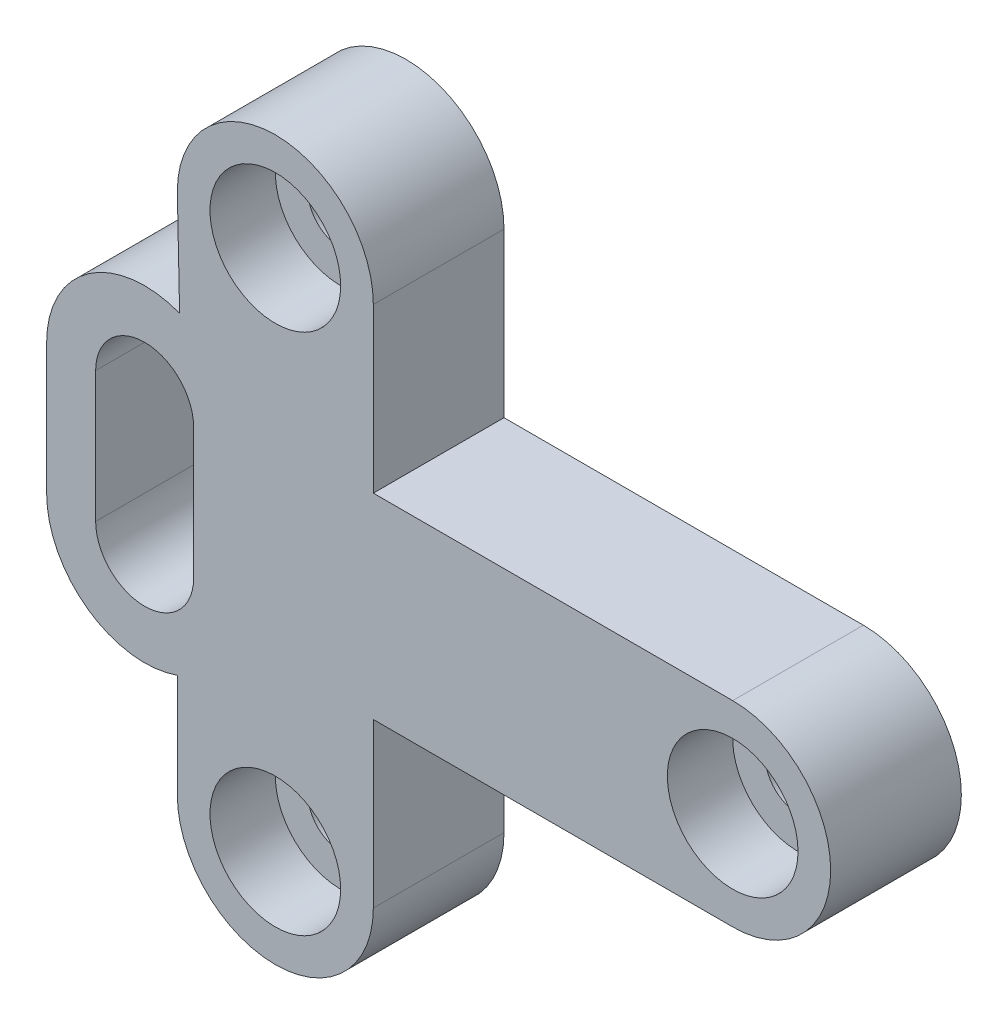
ISO-10303-21;
HEADER;
FILE_DESCRIPTION(('STEP AP214'),'2;1');
FILE_NAME('part.step','',(''),(''),'','','');
FILE_SCHEMA(('AUTOMOTIVE_DESIGN { 1 0 10303 214 1 1 1 1 }'));
ENDSEC;
DATA;
#1=APPLICATION_CONTEXT('core data for automotive mechanical design processes');
#2=APPLICATION_PROTOCOL_DEFINITION('international standard','automotive_design',2000,#1);
#3=PRODUCT_CONTEXT('',#1,'mechanical');
#4=PRODUCT('Part','Part','',(#3));
#5=PRODUCT_RELATED_PRODUCT_CATEGORY('part','',(#4));
#6=PRODUCT_DEFINITION_FORMATION('','',#4);
#7=PRODUCT_DEFINITION_CONTEXT('part definition',#1,'design');
#8=PRODUCT_DEFINITION('design','',#6,#7);
#9=PRODUCT_DEFINITION_SHAPE('','',#8);
#10=(LENGTH_UNIT() NAMED_UNIT(*) SI_UNIT(.MILLI.,.METRE.));
#11=(NAMED_UNIT(*) PLANE_ANGLE_UNIT() SI_UNIT($,.RADIAN.));
#12=(NAMED_UNIT(*) SI_UNIT($,.STERADIAN.) SOLID_ANGLE_UNIT());
#13=UNCERTAINTY_MEASURE_WITH_UNIT(LENGTH_MEASURE(1.E-05),#10,'distance_accuracy_value','');
#14=(GEOMETRIC_REPRESENTATION_CONTEXT(3) GLOBAL_UNCERTAINTY_ASSIGNED_CONTEXT((#13)) GLOBAL_UNIT_ASSIGNED_CONTEXT((#10,
#11,#12)) REPRESENTATION_CONTEXT('',''));
#15=CARTESIAN_POINT('',(0.,0.,0.));
#16=DIRECTION('',(0.,0.,1.));
#17=DIRECTION('',(1.,0.,0.));
#18=AXIS2_PLACEMENT_3D('',#15,#16,#17);
#19=CARTESIAN_POINT('',(-35.0000000000002,-5.34294830600858E-13,20.));
#20=DIRECTION('',(1.,0.,0.));
#21=DIRECTION('',(0.,1.,0.));
#22=AXIS2_PLACEMENT_3D('',#19,#20,#21);
#23=PLANE('',#22);
#24=DIRECTION('',(0.,-1.,0.));
#25=VECTOR('',#24,1.);
#26=CARTESIAN_POINT('',(-35.0000000000002,-5.34294830600858E-13,0.));
#27=LINE('',#26,#25);
#28=CARTESIAN_POINT('',(-35.0000000000003,10.,0.));
#29=VERTEX_POINT('',#28);
#30=CARTESIAN_POINT('',(-35.,-10.,0.));
#31=VERTEX_POINT('',#30);
#32=EDGE_CURVE('E208',#29,#31,#27,.T.);
#33=ORIENTED_EDGE('',*,*,#32,.T.);
#34=DIRECTION('',(0.,0.,-1.));
#35=VECTOR('',#34,1.);
#36=CARTESIAN_POINT('',(-35.,-10.,20.));
#37=LINE('',#36,#35);
#38=CARTESIAN_POINT('',(-35.,-10.,20.));
#39=VERTEX_POINT('',#38);
#40=EDGE_CURVE('E11',#39,#31,#37,.T.);
#41=ORIENTED_EDGE('',*,*,#40,.F.);
#42=DIRECTION('',(0.,-1.,0.));
#43=VECTOR('',#42,1.);
#44=CARTESIAN_POINT('',(-35.0000000000002,-5.34294830600858E-13,20.));
#45=LINE('',#44,#43);
#46=CARTESIAN_POINT('',(-35.0000000000003,10.,20.));
#47=VERTEX_POINT('',#46);
#48=EDGE_CURVE('E278',#47,#39,#45,.T.);
#49=ORIENTED_EDGE('',*,*,#48,.F.);
#50=DIRECTION('',(0.,0.,-1.));
#51=VECTOR('',#50,1.);
#52=CARTESIAN_POINT('',(-35.0000000000003,10.,20.));
#53=LINE('',#52,#51);
#54=EDGE_CURVE('E237',#47,#29,#53,.T.);
#55=ORIENTED_EDGE('',*,*,#54,.T.);
#56=EDGE_LOOP('',(#33,#41,#49,#55));
#57=FACE_BOUND('',#56,.T.);
#58=ADVANCED_FACE('F50',(#57),#23,.F.);
#59=CARTESIAN_POINT('',(-20.,-10.,20.));
#60=DIRECTION('',(0.,0.,-1.));
#61=DIRECTION('',(-1.,0.,0.));
#62=AXIS2_PLACEMENT_3D('',#59,#60,#61);
#63=CYLINDRICAL_SURFACE('',#62,15.);
#64=CARTESIAN_POINT('',(-20.,-10.,0.));
#65=DIRECTION('',(0.,0.,1.));
#66=DIRECTION('',(1.,0.,0.));
#67=AXIS2_PLACEMENT_3D('',#64,#65,#66);
#68=CIRCLE('',#67,15.);
#69=CARTESIAN_POINT('',(-15.,-24.142135623731,0.));
#70=VERTEX_POINT('',#69);
#71=EDGE_CURVE('E211',#31,#70,#68,.T.);
#72=ORIENTED_EDGE('',*,*,#71,.T.);
#73=DIRECTION('',(0.,0.,-1.));
#74=VECTOR('',#73,1.);
#75=CARTESIAN_POINT('',(-15.,-24.142135623731,20.));
#76=LINE('',#75,#74);
#77=CARTESIAN_POINT('',(-15.,-24.142135623731,20.));
#78=VERTEX_POINT('',#77);
#79=EDGE_CURVE('E60',#78,#70,#76,.T.);
#80=ORIENTED_EDGE('',*,*,#79,.F.);
#81=CARTESIAN_POINT('',(-20.,-10.,20.));
#82=DIRECTION('',(0.,0.,1.));
#83=DIRECTION('',(1.,0.,0.));
#84=AXIS2_PLACEMENT_3D('',#81,#82,#83);
#85=CIRCLE('',#84,15.);
#86=EDGE_CURVE('E290',#39,#78,#85,.T.);
#87=ORIENTED_EDGE('',*,*,#86,.F.);
#88=ORIENTED_EDGE('',*,*,#40,.T.);
#89=EDGE_LOOP('',(#72,#80,#87,#88));
#90=FACE_BOUND('',#89,.T.);
#91=ADVANCED_FACE('F335',(#90),#63,.T.);
#92=CARTESIAN_POINT('',(-15.,0.,20.));
#93=DIRECTION('',(-1.,0.,0.));
#94=DIRECTION('',(0.,0.,1.));
#95=AXIS2_PLACEMENT_3D('',#92,#93,#94);
#96=PLANE('',#95);
#97=DIRECTION('',(0.,1.,0.));
#98=VECTOR('',#97,1.);
#99=CARTESIAN_POINT('',(-15.,0.,0.));
#100=LINE('',#99,#98);
#101=CARTESIAN_POINT('',(-15.,-40.,0.));
#102=VERTEX_POINT('',#101);
#103=EDGE_CURVE('E212',#102,#70,#100,.T.);
#104=ORIENTED_EDGE('',*,*,#103,.F.);
#105=DIRECTION('',(0.,0.,-1.));
#106=VECTOR('',#105,1.);
#107=CARTESIAN_POINT('',(-15.,-40.,20.));
#108=LINE('',#107,#106);
#109=CARTESIAN_POINT('',(-15.,-40.,20.));
#110=VERTEX_POINT('',#109);
#111=EDGE_CURVE('E252',#110,#102,#108,.T.);
#112=ORIENTED_EDGE('',*,*,#111,.F.);
#113=DIRECTION('',(0.,1.,0.));
#114=VECTOR('',#113,1.);
#115=CARTESIAN_POINT('',(-15.,0.,20.));
#116=LINE('',#115,#114);
#117=EDGE_CURVE('E289',#110,#78,#116,.T.);
#118=ORIENTED_EDGE('',*,*,#117,.T.);
#119=ORIENTED_EDGE('',*,*,#79,.T.);
#120=EDGE_LOOP('',(#104,#112,#118,#119));
#121=FACE_BOUND('',#120,.T.);
#122=ADVANCED_FACE('F337',(#121),#96,.T.);
#123=CARTESIAN_POINT('',(0.,-40.,20.));
#124=DIRECTION('',(0.,0.,-1.));
#125=DIRECTION('',(-1.,0.,0.));
#126=AXIS2_PLACEMENT_3D('',#123,#124,#125);
#127=CYLINDRICAL_SURFACE('',#126,15.);
#128=CARTESIAN_POINT('',(0.,-40.,0.));
#129=DIRECTION('',(0.,0.,1.));
#130=DIRECTION('',(1.,0.,0.));
#131=AXIS2_PLACEMENT_3D('',#128,#129,#130);
#132=CIRCLE('',#131,15.);
#133=CARTESIAN_POINT('',(15.,-40.,0.));
#134=VERTEX_POINT('',#133);
#135=EDGE_CURVE('E220',#102,#134,#132,.T.);
#136=ORIENTED_EDGE('',*,*,#135,.T.);
#137=DIRECTION('',(0.,0.,-1.));
#138=VECTOR('',#137,1.);
#139=CARTESIAN_POINT('',(15.,-40.,20.));
#140=LINE('',#139,#138);
#141=CARTESIAN_POINT('',(15.,-40.,20.));
#142=VERTEX_POINT('',#141);
#143=EDGE_CURVE('E247',#142,#134,#140,.T.);
#144=ORIENTED_EDGE('',*,*,#143,.F.);
#145=CARTESIAN_POINT('',(0.,-40.,20.));
#146=DIRECTION('',(0.,0.,1.));
#147=DIRECTION('',(1.,0.,0.));
#148=AXIS2_PLACEMENT_3D('',#145,#146,#147);
#149=CIRCLE('',#148,15.);
#150=EDGE_CURVE('E295',#110,#142,#149,.T.);
#151=ORIENTED_EDGE('',*,*,#150,.F.);
#152=ORIENTED_EDGE('',*,*,#111,.T.);
#153=EDGE_LOOP('',(#136,#144,#151,#152));
#154=FACE_BOUND('',#153,.T.);
#155=ADVANCED_FACE('F373',(#154),#127,.T.);
#156=CARTESIAN_POINT('',(15.,0.,20.));
#157=DIRECTION('',(1.,0.,0.));
#158=DIRECTION('',(0.,0.,-1.));
#159=AXIS2_PLACEMENT_3D('',#156,#157,#158);
#160=PLANE('',#159);
#161=DIRECTION('',(0.,-1.,0.));
#162=VECTOR('',#161,1.);
#163=CARTESIAN_POINT('',(15.,0.,0.));
#164=LINE('',#163,#162);
#165=CARTESIAN_POINT('',(15.,-15.,0.));
#166=VERTEX_POINT('',#165);
#167=EDGE_CURVE('E219',#166,#134,#164,.T.);
#168=ORIENTED_EDGE('',*,*,#167,.F.);
#169=DIRECTION('',(0.,0.,-1.));
#170=VECTOR('',#169,1.);
#171=CARTESIAN_POINT('',(15.,-15.,20.));
#172=LINE('',#171,#170);
#173=CARTESIAN_POINT('',(15.,-15.,20.));
#174=VERTEX_POINT('',#173);
#175=EDGE_CURVE('E246',#174,#166,#172,.T.);
#176=ORIENTED_EDGE('',*,*,#175,.F.);
#177=DIRECTION('',(0.,-1.,0.));
#178=VECTOR('',#177,1.);
#179=CARTESIAN_POINT('',(15.,0.,20.));
#180=LINE('',#179,#178);
#181=EDGE_CURVE('E294',#174,#142,#180,.T.);
#182=ORIENTED_EDGE('',*,*,#181,.T.);
#183=ORIENTED_EDGE('',*,*,#143,.T.);
#184=EDGE_LOOP('',(#168,#176,#182,#183));
#185=FACE_BOUND('',#184,.T.);
#186=ADVANCED_FACE('F369',(#185),#160,.T.);
#187=CARTESIAN_POINT('',(0.,-15.,20.));
#188=DIRECTION('',(0.,-1.,0.));
#189=DIRECTION('',(0.,0.,-1.));
#190=AXIS2_PLACEMENT_3D('',#187,#188,#189);
#191=PLANE('',#190);
#192=DIRECTION('',(-1.,0.,0.));
#193=VECTOR('',#192,1.);
#194=CARTESIAN_POINT('',(0.,-15.,0.));
#195=LINE('',#194,#193);
#196=CARTESIAN_POINT('',(70.,-15.,0.));
#197=VERTEX_POINT('',#196);
#198=EDGE_CURVE('E224',#197,#166,#195,.T.);
#199=ORIENTED_EDGE('',*,*,#198,.F.);
#200=DIRECTION('',(0.,0.,-1.));
#201=VECTOR('',#200,1.);
#202=CARTESIAN_POINT('',(70.,-15.,20.));
#203=LINE('',#202,#201);
#204=CARTESIAN_POINT('',(70.,-15.,20.));
#205=VERTEX_POINT('',#204);
#206=EDGE_CURVE('E248',#205,#197,#203,.T.);
#207=ORIENTED_EDGE('',*,*,#206,.F.);
#208=DIRECTION('',(-1.,0.,0.));
#209=VECTOR('',#208,1.);
#210=CARTESIAN_POINT('',(0.,-15.,20.));
#211=LINE('',#210,#209);
#212=EDGE_CURVE('E299',#205,#174,#211,.T.);
#213=ORIENTED_EDGE('',*,*,#212,.T.);
#214=ORIENTED_EDGE('',*,*,#175,.T.);
#215=EDGE_LOOP('',(#199,#207,#213,#214));
#216=FACE_BOUND('',#215,.T.);
#217=ADVANCED_FACE('F364',(#216),#191,.T.);
#218=CARTESIAN_POINT('',(70.,0.,20.));
#219=DIRECTION('',(0.,0.,-1.));
#220=DIRECTION('',(-1.,0.,0.));
#221=AXIS2_PLACEMENT_3D('',#218,#219,#220);
#222=CYLINDRICAL_SURFACE('',#221,15.);
#223=CARTESIAN_POINT('',(70.,0.,0.));
#224=DIRECTION('',(0.,0.,1.));
#225=DIRECTION('',(1.,0.,0.));
#226=AXIS2_PLACEMENT_3D('',#223,#224,#225);
#227=CIRCLE('',#226,15.);
#228=CARTESIAN_POINT('',(70.,15.,0.));
#229=VERTEX_POINT('',#228);
#230=EDGE_CURVE('E228',#197,#229,#227,.T.);
#231=ORIENTED_EDGE('',*,*,#230,.T.);
#232=DIRECTION('',(0.,0.,-1.));
#233=VECTOR('',#232,1.);
#234=CARTESIAN_POINT('',(70.,15.,20.));
#235=LINE('',#234,#233);
#236=CARTESIAN_POINT('',(70.,15.,20.));
#237=VERTEX_POINT('',#236);
#238=EDGE_CURVE('E242',#237,#229,#235,.T.);
#239=ORIENTED_EDGE('',*,*,#238,.F.);
#240=CARTESIAN_POINT('',(70.,0.,20.));
#241=DIRECTION('',(0.,0.,1.));
#242=DIRECTION('',(1.,0.,0.));
#243=AXIS2_PLACEMENT_3D('',#240,#241,#242);
#244=CIRCLE('',#243,15.);
#245=EDGE_CURVE('E296',#205,#237,#244,.T.);
#246=ORIENTED_EDGE('',*,*,#245,.F.);
#247=ORIENTED_EDGE('',*,*,#206,.T.);
#248=EDGE_LOOP('',(#231,#239,#246,#247));
#249=FACE_BOUND('',#248,.T.);
#250=ADVANCED_FACE('F362',(#249),#222,.T.);
#251=CARTESIAN_POINT('',(0.,15.,20.));
#252=DIRECTION('',(0.,-1.,0.));
#253=DIRECTION('',(0.,0.,-1.));
#254=AXIS2_PLACEMENT_3D('',#251,#252,#253);
#255=PLANE('',#254);
#256=DIRECTION('',(-1.,0.,0.));
#257=VECTOR('',#256,1.);
#258=CARTESIAN_POINT('',(0.,15.,0.));
#259=LINE('',#258,#257);
#260=CARTESIAN_POINT('',(15.,15.,0.));
#261=VERTEX_POINT('',#260);
#262=EDGE_CURVE('E227',#229,#261,#259,.T.);
#263=ORIENTED_EDGE('',*,*,#262,.T.);
#264=DIRECTION('',(0.,0.,-1.));
#265=VECTOR('',#264,1.);
#266=CARTESIAN_POINT('',(15.,15.,20.));
#267=LINE('',#266,#265);
#268=CARTESIAN_POINT('',(15.,15.,20.));
#269=VERTEX_POINT('',#268);
#270=EDGE_CURVE('E238',#269,#261,#267,.T.);
#271=ORIENTED_EDGE('',*,*,#270,.F.);
#272=DIRECTION('',(-1.,0.,0.));
#273=VECTOR('',#272,1.);
#274=CARTESIAN_POINT('',(0.,15.,20.));
#275=LINE('',#274,#273);
#276=EDGE_CURVE('E305',#237,#269,#275,.T.);
#277=ORIENTED_EDGE('',*,*,#276,.F.);
#278=ORIENTED_EDGE('',*,*,#238,.T.);
#279=EDGE_LOOP('',(#263,#271,#277,#278));
#280=FACE_BOUND('',#279,.T.);
#281=ADVANCED_FACE('F310',(#280),#255,.F.);
#282=CARTESIAN_POINT('',(15.,0.,20.));
#283=DIRECTION('',(-1.,0.,0.));
#284=DIRECTION('',(0.,0.,1.));
#285=AXIS2_PLACEMENT_3D('',#282,#283,#284);
#286=PLANE('',#285);
#287=DIRECTION('',(0.,1.,0.));
#288=VECTOR('',#287,1.);
#289=CARTESIAN_POINT('',(15.,0.,0.));
#290=LINE('',#289,#288);
#291=CARTESIAN_POINT('',(15.,40.,0.));
#292=VERTEX_POINT('',#291);
#293=EDGE_CURVE('E226',#261,#292,#290,.T.);
#294=ORIENTED_EDGE('',*,*,#293,.T.);
#295=DIRECTION('',(0.,0.,-1.));
#296=VECTOR('',#295,1.);
#297=CARTESIAN_POINT('',(15.,40.,20.));
#298=LINE('',#297,#296);
#299=CARTESIAN_POINT('',(15.,40.,20.));
#300=VERTEX_POINT('',#299);
#301=EDGE_CURVE('E188',#300,#292,#298,.T.);
#302=ORIENTED_EDGE('',*,*,#301,.F.);
#303=DIRECTION('',(0.,1.,0.));
#304=VECTOR('',#303,1.);
#305=CARTESIAN_POINT('',(15.,0.,20.));
#306=LINE('',#305,#304);
#307=EDGE_CURVE('E180',#269,#300,#306,.T.);
#308=ORIENTED_EDGE('',*,*,#307,.F.);
#309=ORIENTED_EDGE('',*,*,#270,.T.);
#310=EDGE_LOOP('',(#294,#302,#308,#309));
#311=FACE_BOUND('',#310,.T.);
#312=ADVANCED_FACE('F311',(#311),#286,.F.);
#313=CARTESIAN_POINT('',(0.,40.,20.));
#314=DIRECTION('',(0.,0.,-1.));
#315=DIRECTION('',(-1.,0.,0.));
#316=AXIS2_PLACEMENT_3D('',#313,#314,#315);
#317=CYLINDRICAL_SURFACE('',#316,15.0000000000002);
#318=CARTESIAN_POINT('',(0.,40.,0.));
#319=DIRECTION('',(0.,0.,1.));
#320=DIRECTION('',(1.,0.,0.));
#321=AXIS2_PLACEMENT_3D('',#318,#319,#320);
#322=CIRCLE('',#321,15.0000000000002);
#323=CARTESIAN_POINT('',(-15.,40.,0.));
#324=VERTEX_POINT('',#323);
#325=EDGE_CURVE('E183',#292,#324,#322,.T.);
#326=ORIENTED_EDGE('',*,*,#325,.T.);
#327=DIRECTION('',(0.,0.,-1.));
#328=VECTOR('',#327,1.);
#329=CARTESIAN_POINT('',(-15.,40.,20.));
#330=LINE('',#329,#328);
#331=CARTESIAN_POINT('',(-15.,40.,20.));
#332=VERTEX_POINT('',#331);
#333=EDGE_CURVE('E185',#332,#324,#330,.T.);
#334=ORIENTED_EDGE('',*,*,#333,.F.);
#335=CARTESIAN_POINT('',(0.,40.,20.));
#336=DIRECTION('',(0.,0.,1.));
#337=DIRECTION('',(1.,0.,0.));
#338=AXIS2_PLACEMENT_3D('',#335,#336,#337);
#339=CIRCLE('',#338,15.0000000000002);
#340=EDGE_CURVE('E173',#300,#332,#339,.T.);
#341=ORIENTED_EDGE('',*,*,#340,.F.);
#342=ORIENTED_EDGE('',*,*,#301,.T.);
#343=EDGE_LOOP('',(#326,#334,#341,#342));
#344=FACE_BOUND('',#343,.T.);
#345=ADVANCED_FACE('F181',(#344),#317,.T.);
#346=CARTESIAN_POINT('',(-14.111624571702,-0.310992603092202,20.));
#347=DIRECTION('',(0.999757250727962,0.0220326942716201,0.));
#348=DIRECTION('',(-0.0220326942716201,0.999757250727962,0.));
#349=AXIS2_PLACEMENT_3D('',#346,#347,#348);
#350=PLANE('',#349);
#351=DIRECTION('',(0.0220326942716201,-0.999757250727962,0.));
#352=VECTOR('',#351,1.);
#353=CARTESIAN_POINT('',(-14.111624571702,-0.310992603092202,0.));
#354=LINE('',#353,#352);
#355=CARTESIAN_POINT('',(-14.6476686534038,24.0125853844407,0.));
#356=VERTEX_POINT('',#355);
#357=EDGE_CURVE('E120',#324,#356,#354,.T.);
#358=ORIENTED_EDGE('',*,*,#357,.T.);
#359=DIRECTION('',(0.,0.,-1.));
#360=VECTOR('',#359,1.);
#361=CARTESIAN_POINT('',(-14.6476686534038,24.0125853844407,20.));
#362=LINE('',#361,#360);
#363=CARTESIAN_POINT('',(-14.6476686534038,24.0125853844407,20.));
#364=VERTEX_POINT('',#363);
#365=EDGE_CURVE('E189',#364,#356,#362,.T.);
#366=ORIENTED_EDGE('',*,*,#365,.F.);
#367=DIRECTION('',(0.0220326942716201,-0.999757250727962,0.));
#368=VECTOR('',#367,1.);
#369=CARTESIAN_POINT('',(-14.111624571702,-0.310992603092202,20.));
#370=LINE('',#369,#368);
#371=EDGE_CURVE('E171',#332,#364,#370,.T.);
#372=ORIENTED_EDGE('',*,*,#371,.F.);
#373=ORIENTED_EDGE('',*,*,#333,.T.);
#374=EDGE_LOOP('',(#358,#366,#372,#373));
#375=FACE_BOUND('',#374,.T.);
#376=ADVANCED_FACE('F190',(#375),#350,.F.);
#377=CARTESIAN_POINT('',(-20.,-10.,20.));
#378=DIRECTION('',(0.,0.,-1.));
#379=DIRECTION('',(-1.,0.,0.));
#380=AXIS2_PLACEMENT_3D('',#377,#378,#379);
#381=CYLINDRICAL_SURFACE('',#380,7.5);
#382=CARTESIAN_POINT('',(-20.,-10.,0.));
#383=DIRECTION('',(0.,0.,1.));
#384=DIRECTION('',(1.,0.,0.));
#385=AXIS2_PLACEMENT_3D('',#382,#383,#384);
#386=CIRCLE('',#385,7.5);
#387=CARTESIAN_POINT('',(-27.5,-10.,0.));
#388=VERTEX_POINT('',#387);
#389=CARTESIAN_POINT('',(-12.5,-10.,0.));
#390=VERTEX_POINT('',#389);
#391=EDGE_CURVE('E192',#388,#390,#386,.T.);
#392=ORIENTED_EDGE('',*,*,#391,.F.);
#393=DIRECTION('',(0.,0.,-1.));
#394=VECTOR('',#393,1.);
#395=CARTESIAN_POINT('',(-27.5,-10.,20.));
#396=LINE('',#395,#394);
#397=CARTESIAN_POINT('',(-27.5,-10.,20.));
#398=VERTEX_POINT('',#397);
#399=EDGE_CURVE('E51',#398,#388,#396,.T.);
#400=ORIENTED_EDGE('',*,*,#399,.F.);
#401=CARTESIAN_POINT('',(-20.,-10.,20.));
#402=DIRECTION('',(0.,0.,1.));
#403=DIRECTION('',(1.,0.,0.));
#404=AXIS2_PLACEMENT_3D('',#401,#402,#403);
#405=CIRCLE('',#404,7.5);
#406=CARTESIAN_POINT('',(-12.5,-10.,20.));
#407=VERTEX_POINT('',#406);
#408=EDGE_CURVE('E232',#398,#407,#405,.T.);
#409=ORIENTED_EDGE('',*,*,#408,.T.);
#410=DIRECTION('',(0.,0.,-1.));
#411=VECTOR('',#410,1.);
#412=CARTESIAN_POINT('',(-12.5,-10.,20.));
#413=LINE('',#412,#411);
#414=EDGE_CURVE('E193',#407,#390,#413,.T.);
#415=ORIENTED_EDGE('',*,*,#414,.T.);
#416=EDGE_LOOP('',(#392,#400,#409,#415));
#417=FACE_BOUND('',#416,.T.);
#418=ADVANCED_FACE('F47',(#417),#381,.F.);
#419=CARTESIAN_POINT('',(-27.5,0.,20.));
#420=DIRECTION('',(1.,0.,0.));
#421=DIRECTION('',(0.,0.,-1.));
#422=AXIS2_PLACEMENT_3D('',#419,#420,#421);
#423=PLANE('',#422);
#424=DIRECTION('',(0.,-1.,0.));
#425=VECTOR('',#424,1.);
#426=CARTESIAN_POINT('',(-27.5,0.,0.));
#427=LINE('',#426,#425);
#428=CARTESIAN_POINT('',(-27.5,10.,0.));
#429=VERTEX_POINT('',#428);
#430=EDGE_CURVE('E196',#429,#388,#427,.T.);
#431=ORIENTED_EDGE('',*,*,#430,.F.);
#432=DIRECTION('',(0.,0.,-1.));
#433=VECTOR('',#432,1.);
#434=CARTESIAN_POINT('',(-27.5,10.,20.));
#435=LINE('',#434,#433);
#436=CARTESIAN_POINT('',(-27.5,10.,20.));
#437=VERTEX_POINT('',#436);
#438=EDGE_CURVE('E260',#437,#429,#435,.T.);
#439=ORIENTED_EDGE('',*,*,#438,.F.);
#440=DIRECTION('',(0.,-1.,0.));
#441=VECTOR('',#440,1.);
#442=CARTESIAN_POINT('',(-27.5,0.,20.));
#443=LINE('',#442,#441);
#444=EDGE_CURVE('E266',#437,#398,#443,.T.);
#445=ORIENTED_EDGE('',*,*,#444,.T.);
#446=ORIENTED_EDGE('',*,*,#399,.T.);
#447=EDGE_LOOP('',(#431,#439,#445,#446));
#448=FACE_BOUND('',#447,.T.);
#449=ADVANCED_FACE('F262',(#448),#423,.T.);
#450=CARTESIAN_POINT('',(-20.,10.,20.));
#451=DIRECTION('',(0.,0.,-1.));
#452=DIRECTION('',(-1.,0.,0.));
#453=AXIS2_PLACEMENT_3D('',#450,#451,#452);
#454=CYLINDRICAL_SURFACE('',#453,7.5);
#455=CARTESIAN_POINT('',(-20.,10.,0.));
#456=DIRECTION('',(0.,0.,1.));
#457=DIRECTION('',(1.,0.,0.));
#458=AXIS2_PLACEMENT_3D('',#455,#456,#457);
#459=CIRCLE('',#458,7.5);
#460=CARTESIAN_POINT('',(-12.5,10.,0.));
#461=VERTEX_POINT('',#460);
#462=EDGE_CURVE('E205',#461,#429,#459,.T.);
#463=ORIENTED_EDGE('',*,*,#462,.F.);
#464=DIRECTION('',(0.,0.,-1.));
#465=VECTOR('',#464,1.);
#466=CARTESIAN_POINT('',(-12.5,10.,20.));
#467=LINE('',#466,#465);
#468=CARTESIAN_POINT('',(-12.5,10.,20.));
#469=VERTEX_POINT('',#468);
#470=EDGE_CURVE('E258',#469,#461,#467,.T.);
#471=ORIENTED_EDGE('',*,*,#470,.F.);
#472=CARTESIAN_POINT('',(-20.,10.,20.));
#473=DIRECTION('',(0.,0.,1.));
#474=DIRECTION('',(1.,0.,0.));
#475=AXIS2_PLACEMENT_3D('',#472,#473,#474);
#476=CIRCLE('',#475,7.5);
#477=EDGE_CURVE('E274',#469,#437,#476,.T.);
#478=ORIENTED_EDGE('',*,*,#477,.T.);
#479=ORIENTED_EDGE('',*,*,#438,.T.);
#480=EDGE_LOOP('',(#463,#471,#478,#479));
#481=FACE_BOUND('',#480,.T.);
#482=ADVANCED_FACE('F275',(#481),#454,.F.);
#483=CARTESIAN_POINT('',(-12.5,0.,20.));
#484=DIRECTION('',(1.,0.,0.));
#485=DIRECTION('',(0.,0.,-1.));
#486=AXIS2_PLACEMENT_3D('',#483,#484,#485);
#487=PLANE('',#486);
#488=DIRECTION('',(0.,-1.,0.));
#489=VECTOR('',#488,1.);
#490=CARTESIAN_POINT('',(-12.5,0.,0.));
#491=LINE('',#490,#489);
#492=EDGE_CURVE('E202',#461,#390,#491,.T.);
#493=ORIENTED_EDGE('',*,*,#492,.T.);
#494=ORIENTED_EDGE('',*,*,#414,.F.);
#495=DIRECTION('',(0.,-1.,0.));
#496=VECTOR('',#495,1.);
#497=CARTESIAN_POINT('',(-12.5,0.,20.));
#498=LINE('',#497,#496);
#499=EDGE_CURVE('E280',#469,#407,#498,.T.);
#500=ORIENTED_EDGE('',*,*,#499,.F.);
#501=ORIENTED_EDGE('',*,*,#470,.T.);
#502=EDGE_LOOP('',(#493,#494,#500,#501));
#503=FACE_BOUND('',#502,.T.);
#504=ADVANCED_FACE('F279',(#503),#487,.F.);
#505=CARTESIAN_POINT('',(-20.,10.,20.));
#506=DIRECTION('',(0.,0.,-1.));
#507=DIRECTION('',(-1.,0.,0.));
#508=AXIS2_PLACEMENT_3D('',#505,#506,#507);
#509=CYLINDRICAL_SURFACE('',#508,15.0000000000001);
#510=CARTESIAN_POINT('',(-20.,10.,0.));
#511=DIRECTION('',(0.,0.,1.));
#512=DIRECTION('',(1.,0.,0.));
#513=AXIS2_PLACEMENT_3D('',#510,#511,#512);
#514=CIRCLE('',#513,15.0000000000001);
#515=EDGE_CURVE('E122',#356,#29,#514,.T.);
#516=ORIENTED_EDGE('',*,*,#515,.T.);
#517=ORIENTED_EDGE('',*,*,#54,.F.);
#518=CARTESIAN_POINT('',(-20.,10.,20.));
#519=DIRECTION('',(0.,0.,1.));
#520=DIRECTION('',(1.,0.,0.));
#521=AXIS2_PLACEMENT_3D('',#518,#519,#520);
#522=CIRCLE('',#521,15.0000000000001);
#523=EDGE_CURVE('E68',#364,#47,#522,.T.);
#524=ORIENTED_EDGE('',*,*,#523,.F.);
#525=ORIENTED_EDGE('',*,*,#365,.T.);
#526=EDGE_LOOP('',(#516,#517,#524,#525));
#527=FACE_BOUND('',#526,.T.);
#528=ADVANCED_FACE('F318',(#527),#509,.T.);
#529=CARTESIAN_POINT('',(0.,0.,20.));
#530=DIRECTION('',(0.,0.,1.));
#531=DIRECTION('',(1.,0.,0.));
#532=AXIS2_PLACEMENT_3D('',#529,#530,#531);
#533=PLANE('',#532);
#534=CARTESIAN_POINT('',(0.,40.,20.));
#535=DIRECTION('',(0.,0.,1.));
#536=DIRECTION('',(1.,0.,0.));
#537=AXIS2_PLACEMENT_3D('',#534,#535,#536);
#538=CIRCLE('',#537,10.);
#539=CARTESIAN_POINT('',(10.,40.,20.));
#540=VERTEX_POINT('',#539);
#541=EDGE_CURVE('E688',#540,#540,#538,.T.);
#542=ORIENTED_EDGE('',*,*,#541,.F.);
#543=EDGE_LOOP('',(#542));
#544=FACE_BOUND('',#543,.T.);
#545=CARTESIAN_POINT('',(0.,-40.,20.));
#546=DIRECTION('',(0.,0.,1.));
#547=DIRECTION('',(1.,0.,0.));
#548=AXIS2_PLACEMENT_3D('',#545,#546,#547);
#549=CIRCLE('',#548,10.);
#550=CARTESIAN_POINT('',(10.,-40.,20.));
#551=VERTEX_POINT('',#550);
#552=EDGE_CURVE('E692',#551,#551,#549,.T.);
#553=ORIENTED_EDGE('',*,*,#552,.F.);
#554=EDGE_LOOP('',(#553));
#555=FACE_BOUND('',#554,.T.);
#556=CARTESIAN_POINT('',(70.,0.,20.));
#557=DIRECTION('',(0.,0.,1.));
#558=DIRECTION('',(1.,0.,0.));
#559=AXIS2_PLACEMENT_3D('',#556,#557,#558);
#560=CIRCLE('',#559,10.);
#561=CARTESIAN_POINT('',(80.,0.,20.));
#562=VERTEX_POINT('',#561);
#563=EDGE_CURVE('E696',#562,#562,#560,.T.);
#564=ORIENTED_EDGE('',*,*,#563,.F.);
#565=EDGE_LOOP('',(#564));
#566=FACE_BOUND('',#565,.T.);
#567=ORIENTED_EDGE('',*,*,#408,.F.);
#568=ORIENTED_EDGE('',*,*,#444,.F.);
#569=ORIENTED_EDGE('',*,*,#477,.F.);
#570=ORIENTED_EDGE('',*,*,#499,.T.);
#571=EDGE_LOOP('',(#567,#568,#569,#570));
#572=FACE_BOUND('',#571,.T.);
#573=ORIENTED_EDGE('',*,*,#48,.T.);
#574=ORIENTED_EDGE('',*,*,#86,.T.);
#575=ORIENTED_EDGE('',*,*,#117,.F.);
#576=ORIENTED_EDGE('',*,*,#150,.T.);
#577=ORIENTED_EDGE('',*,*,#181,.F.);
#578=ORIENTED_EDGE('',*,*,#212,.F.);
#579=ORIENTED_EDGE('',*,*,#245,.T.);
#580=ORIENTED_EDGE('',*,*,#276,.T.);
#581=ORIENTED_EDGE('',*,*,#307,.T.);
#582=ORIENTED_EDGE('',*,*,#340,.T.);
#583=ORIENTED_EDGE('',*,*,#371,.T.);
#584=ORIENTED_EDGE('',*,*,#523,.T.);
#585=EDGE_LOOP('',(#573,#574,#575,#576,#577,#578,#579,#580,#581,#582,#583,#584));
#586=FACE_BOUND('',#585,.T.);
#587=ADVANCED_FACE('F172',(#544,#555,#566,#572,#586),#533,.T.);
#588=CARTESIAN_POINT('',(0.,0.,0.));
#589=DIRECTION('',(0.,0.,1.));
#590=DIRECTION('',(1.,0.,0.));
#591=AXIS2_PLACEMENT_3D('',#588,#589,#590);
#592=PLANE('',#591);
#593=CARTESIAN_POINT('',(0.,40.,0.));
#594=DIRECTION('',(0.,0.,1.));
#595=DIRECTION('',(1.,0.,0.));
#596=AXIS2_PLACEMENT_3D('',#593,#594,#595);
#597=CIRCLE('',#596,5.);
#598=CARTESIAN_POINT('',(5.,40.,0.));
#599=VERTEX_POINT('',#598);
#600=EDGE_CURVE('E669',#599,#599,#597,.T.);
#601=ORIENTED_EDGE('',*,*,#600,.T.);
#602=EDGE_LOOP('',(#601));
#603=FACE_BOUND('',#602,.T.);
#604=CARTESIAN_POINT('',(0.,-40.,0.));
#605=DIRECTION('',(0.,0.,1.));
#606=DIRECTION('',(1.,0.,0.));
#607=AXIS2_PLACEMENT_3D('',#604,#605,#606);
#608=CIRCLE('',#607,5.);
#609=CARTESIAN_POINT('',(5.,-40.,0.));
#610=VERTEX_POINT('',#609);
#611=EDGE_CURVE('E673',#610,#610,#608,.T.);
#612=ORIENTED_EDGE('',*,*,#611,.T.);
#613=EDGE_LOOP('',(#612));
#614=FACE_BOUND('',#613,.T.);
#615=CARTESIAN_POINT('',(70.,0.,0.));
#616=DIRECTION('',(0.,0.,1.));
#617=DIRECTION('',(1.,0.,0.));
#618=AXIS2_PLACEMENT_3D('',#615,#616,#617);
#619=CIRCLE('',#618,5.);
#620=CARTESIAN_POINT('',(75.,0.,0.));
#621=VERTEX_POINT('',#620);
#622=EDGE_CURVE('E674',#621,#621,#619,.T.);
#623=ORIENTED_EDGE('',*,*,#622,.T.);
#624=EDGE_LOOP('',(#623));
#625=FACE_BOUND('',#624,.T.);
#626=ORIENTED_EDGE('',*,*,#391,.T.);
#627=ORIENTED_EDGE('',*,*,#492,.F.);
#628=ORIENTED_EDGE('',*,*,#462,.T.);
#629=ORIENTED_EDGE('',*,*,#430,.T.);
#630=EDGE_LOOP('',(#626,#627,#628,#629));
#631=FACE_BOUND('',#630,.T.);
#632=ORIENTED_EDGE('',*,*,#32,.F.);
#633=ORIENTED_EDGE('',*,*,#515,.F.);
#634=ORIENTED_EDGE('',*,*,#357,.F.);
#635=ORIENTED_EDGE('',*,*,#325,.F.);
#636=ORIENTED_EDGE('',*,*,#293,.F.);
#637=ORIENTED_EDGE('',*,*,#262,.F.);
#638=ORIENTED_EDGE('',*,*,#230,.F.);
#639=ORIENTED_EDGE('',*,*,#198,.T.);
#640=ORIENTED_EDGE('',*,*,#167,.T.);
#641=ORIENTED_EDGE('',*,*,#135,.F.);
#642=ORIENTED_EDGE('',*,*,#103,.T.);
#643=ORIENTED_EDGE('',*,*,#71,.F.);
#644=EDGE_LOOP('',(#632,#633,#634,#635,#636,#637,#638,#639,#640,#641,#642,#643));
#645=FACE_BOUND('',#644,.T.);
#646=ADVANCED_FACE('F269',(#603,#614,#625,#631,#645),#592,.F.);
#647=CARTESIAN_POINT('',(70.,0.,10.));
#648=DIRECTION('',(0.,0.,1.));
#649=DIRECTION('',(1.,0.,0.));
#650=AXIS2_PLACEMENT_3D('',#647,#648,#649);
#651=CYLINDRICAL_SURFACE('',#650,10.);
#652=CARTESIAN_POINT('',(70.,0.,10.));
#653=DIRECTION('',(0.,0.,1.));
#654=DIRECTION('',(1.,0.,0.));
#655=AXIS2_PLACEMENT_3D('',#652,#653,#654);
#656=CIRCLE('',#655,10.);
#657=CARTESIAN_POINT('',(80.,0.,10.));
#658=VERTEX_POINT('',#657);
#659=EDGE_CURVE('E694',#658,#658,#656,.T.);
#660=ORIENTED_EDGE('',*,*,#659,.F.);
#661=EDGE_LOOP('',(#660));
#662=FACE_BOUND('',#661,.T.);
#663=ORIENTED_EDGE('',*,*,#563,.T.);
#664=EDGE_LOOP('',(#663));
#665=FACE_BOUND('',#664,.T.);
#666=ADVANCED_FACE('F473',(#662,#665),#651,.F.);
#667=CARTESIAN_POINT('',(70.,0.,10.));
#668=DIRECTION('',(0.,0.,1.));
#669=DIRECTION('',(1.,0.,0.));
#670=AXIS2_PLACEMENT_3D('',#667,#668,#669);
#671=PLANE('',#670);
#672=CARTESIAN_POINT('',(70.,0.,10.));
#673=DIRECTION('',(0.,0.,1.));
#674=DIRECTION('',(1.,0.,0.));
#675=AXIS2_PLACEMENT_3D('',#672,#673,#674);
#676=CIRCLE('',#675,5.);
#677=CARTESIAN_POINT('',(75.,0.,10.));
#678=VERTEX_POINT('',#677);
#679=EDGE_CURVE('E677',#678,#678,#676,.T.);
#680=ORIENTED_EDGE('',*,*,#679,.F.);
#681=EDGE_LOOP('',(#680));
#682=FACE_BOUND('',#681,.T.);
#683=ORIENTED_EDGE('',*,*,#659,.T.);
#684=EDGE_LOOP('',(#683));
#685=FACE_BOUND('',#684,.T.);
#686=ADVANCED_FACE('F474',(#682,#685),#671,.T.);
#687=CARTESIAN_POINT('',(0.,-40.,10.));
#688=DIRECTION('',(0.,0.,1.));
#689=DIRECTION('',(1.,0.,0.));
#690=AXIS2_PLACEMENT_3D('',#687,#688,#689);
#691=CYLINDRICAL_SURFACE('',#690,10.);
#692=CARTESIAN_POINT('',(0.,-40.,10.));
#693=DIRECTION('',(0.,0.,1.));
#694=DIRECTION('',(1.,0.,0.));
#695=AXIS2_PLACEMENT_3D('',#692,#693,#694);
#696=CIRCLE('',#695,10.);
#697=CARTESIAN_POINT('',(10.,-40.,10.));
#698=VERTEX_POINT('',#697);
#699=EDGE_CURVE('E689',#698,#698,#696,.T.);
#700=ORIENTED_EDGE('',*,*,#699,.F.);
#701=EDGE_LOOP('',(#700));
#702=FACE_BOUND('',#701,.T.);
#703=ORIENTED_EDGE('',*,*,#552,.T.);
#704=EDGE_LOOP('',(#703));
#705=FACE_BOUND('',#704,.T.);
#706=ADVANCED_FACE('F486',(#702,#705),#691,.F.);
#707=CARTESIAN_POINT('',(0.,-40.,10.));
#708=DIRECTION('',(0.,0.,1.));
#709=DIRECTION('',(1.,0.,0.));
#710=AXIS2_PLACEMENT_3D('',#707,#708,#709);
#711=PLANE('',#710);
#712=CARTESIAN_POINT('',(0.,-40.,10.));
#713=DIRECTION('',(0.,0.,1.));
#714=DIRECTION('',(1.,0.,0.));
#715=AXIS2_PLACEMENT_3D('',#712,#713,#714);
#716=CIRCLE('',#715,5.);
#717=CARTESIAN_POINT('',(5.,-40.,10.));
#718=VERTEX_POINT('',#717);
#719=EDGE_CURVE('E672',#718,#718,#716,.T.);
#720=ORIENTED_EDGE('',*,*,#719,.F.);
#721=EDGE_LOOP('',(#720));
#722=FACE_BOUND('',#721,.T.);
#723=ORIENTED_EDGE('',*,*,#699,.T.);
#724=EDGE_LOOP('',(#723));
#725=FACE_BOUND('',#724,.T.);
#726=ADVANCED_FACE('F497',(#722,#725),#711,.T.);
#727=CARTESIAN_POINT('',(0.,40.,10.));
#728=DIRECTION('',(0.,0.,1.));
#729=DIRECTION('',(1.,0.,0.));
#730=AXIS2_PLACEMENT_3D('',#727,#728,#729);
#731=CYLINDRICAL_SURFACE('',#730,10.);
#732=CARTESIAN_POINT('',(0.,40.,10.));
#733=DIRECTION('',(0.,0.,1.));
#734=DIRECTION('',(1.,0.,0.));
#735=AXIS2_PLACEMENT_3D('',#732,#733,#734);
#736=CIRCLE('',#735,10.);
#737=CARTESIAN_POINT('',(10.,40.,10.));
#738=VERTEX_POINT('',#737);
#739=EDGE_CURVE('E200',#738,#738,#736,.T.);
#740=ORIENTED_EDGE('',*,*,#739,.F.);
#741=EDGE_LOOP('',(#740));
#742=FACE_BOUND('',#741,.T.);
#743=ORIENTED_EDGE('',*,*,#541,.T.);
#744=EDGE_LOOP('',(#743));
#745=FACE_BOUND('',#744,.T.);
#746=ADVANCED_FACE('F510',(#742,#745),#731,.F.);
#747=CARTESIAN_POINT('',(0.,40.,10.));
#748=DIRECTION('',(0.,0.,1.));
#749=DIRECTION('',(1.,0.,0.));
#750=AXIS2_PLACEMENT_3D('',#747,#748,#749);
#751=PLANE('',#750);
#752=CARTESIAN_POINT('',(0.,40.,10.));
#753=DIRECTION('',(0.,0.,1.));
#754=DIRECTION('',(1.,0.,0.));
#755=AXIS2_PLACEMENT_3D('',#752,#753,#754);
#756=CIRCLE('',#755,5.);
#757=CARTESIAN_POINT('',(5.,40.,10.));
#758=VERTEX_POINT('',#757);
#759=EDGE_CURVE('E705',#758,#758,#756,.T.);
#760=ORIENTED_EDGE('',*,*,#759,.F.);
#761=EDGE_LOOP('',(#760));
#762=FACE_BOUND('',#761,.T.);
#763=ORIENTED_EDGE('',*,*,#739,.T.);
#764=EDGE_LOOP('',(#763));
#765=FACE_BOUND('',#764,.T.);
#766=ADVANCED_FACE('F519',(#762,#765),#751,.T.);
#767=CARTESIAN_POINT('',(70.,0.,0.));
#768=DIRECTION('',(0.,0.,1.));
#769=DIRECTION('',(1.,0.,0.));
#770=AXIS2_PLACEMENT_3D('',#767,#768,#769);
#771=CYLINDRICAL_SURFACE('',#770,5.);
#772=ORIENTED_EDGE('',*,*,#622,.F.);
#773=EDGE_LOOP('',(#772));
#774=FACE_BOUND('',#773,.T.);
#775=ORIENTED_EDGE('',*,*,#679,.T.);
#776=EDGE_LOOP('',(#775));
#777=FACE_BOUND('',#776,.T.);
#778=ADVANCED_FACE('F527',(#774,#777),#771,.F.);
#779=CARTESIAN_POINT('',(0.,-40.,0.));
#780=DIRECTION('',(0.,0.,1.));
#781=DIRECTION('',(1.,0.,0.));
#782=AXIS2_PLACEMENT_3D('',#779,#780,#781);
#783=CYLINDRICAL_SURFACE('',#782,5.);
#784=ORIENTED_EDGE('',*,*,#611,.F.);
#785=EDGE_LOOP('',(#784));
#786=FACE_BOUND('',#785,.T.);
#787=ORIENTED_EDGE('',*,*,#719,.T.);
#788=EDGE_LOOP('',(#787));
#789=FACE_BOUND('',#788,.T.);
#790=ADVANCED_FACE('F536',(#786,#789),#783,.F.);
#791=CARTESIAN_POINT('',(0.,40.,0.));
#792=DIRECTION('',(0.,0.,1.));
#793=DIRECTION('',(1.,0.,0.));
#794=AXIS2_PLACEMENT_3D('',#791,#792,#793);
#795=CYLINDRICAL_SURFACE('',#794,5.);
#796=ORIENTED_EDGE('',*,*,#600,.F.);
#797=EDGE_LOOP('',(#796));
#798=FACE_BOUND('',#797,.T.);
#799=ORIENTED_EDGE('',*,*,#759,.T.);
#800=EDGE_LOOP('',(#799));
#801=FACE_BOUND('',#800,.T.);
#802=ADVANCED_FACE('F546',(#798,#801),#795,.F.);
#803=CLOSED_SHELL('',(#58,#91,#122,#155,#186,#217,#250,#281,#312,#345,#376,#418,#449,#482,#504,
#528,#587,#646,#666,#686,#706,#726,#746,#766,#778,#790,#802));
#804=MANIFOLD_SOLID_BREP('B2',#803);
#805=ADVANCED_BREP_SHAPE_REPRESENTATION('',(#18,#804),#14);
#806=SHAPE_DEFINITION_REPRESENTATION(#9,#805);
ENDSEC;
END-ISO-10303-21;
